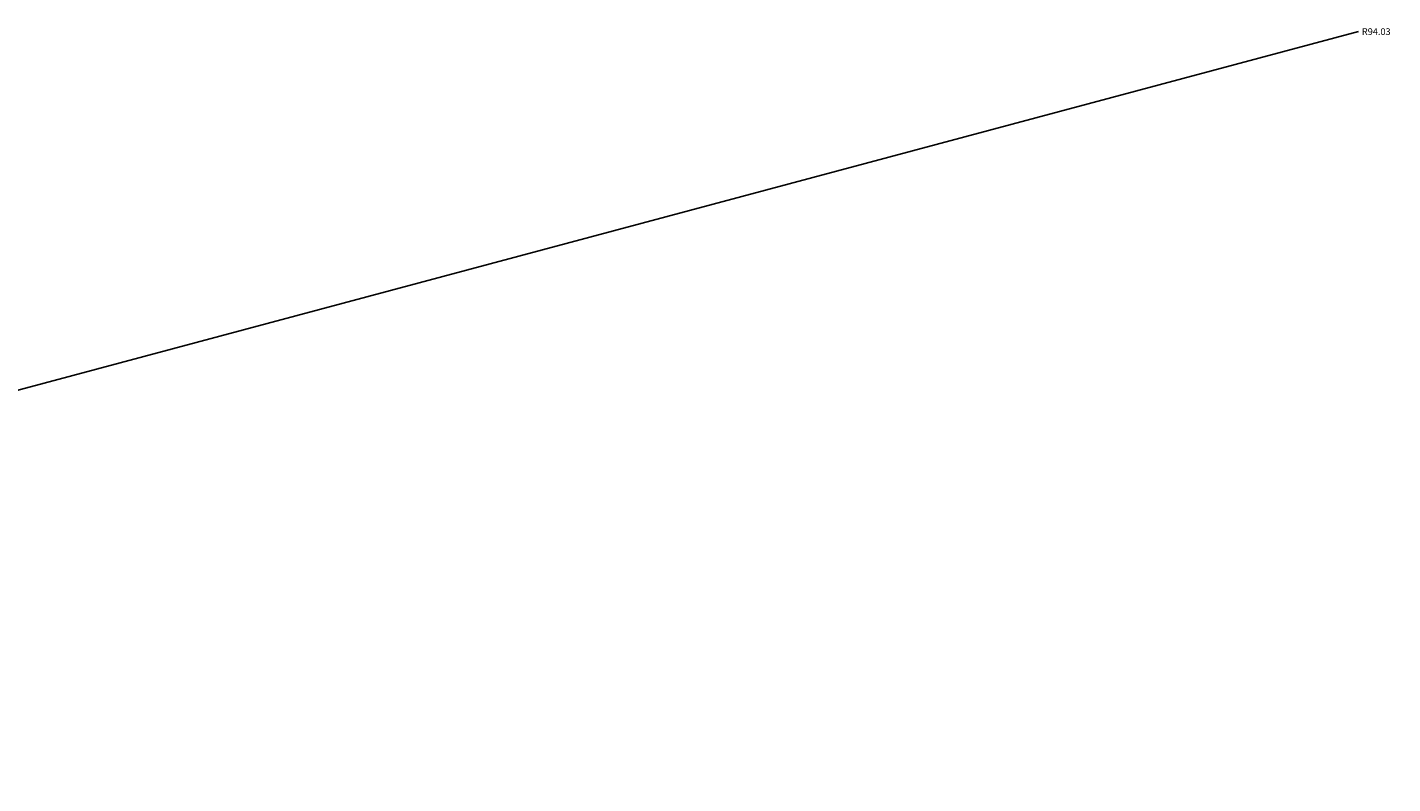
# Model space of a CAD drawing. Units: inches. Extents: x -12 to 334, y -10 to 186.
# Tile 77 of 77: x 297 to 334, y 111 to 131. Entities that reach past the tile are written whole.
import ezdxf

# ---------------------------------------------------------------- set-up
doc = ezdxf.new("R2010")
doc.units = ezdxf.units.IN
doc.header["$MEASUREMENT"] = 0
doc.layers.add('M-DIMS', color=2, linetype='Continuous', lineweight=18)
doc.styles.get("Standard").update_dxf_attribs({"font": 'arial.ttf'})
doc.dimstyles.get("Standard").update_dxf_attribs({"dimtxt": 0.18, "dimasz": 0.18, "dimexe": 0.18, "dimexo": 0.0625, "dimgap": 0.09, "dimtad": 0, "dimtih": 1, "dimtoh": 1, "dimdec": 4, "dimzin": 0, "dimdsep": 46, "dimtxsty": 'Standard', "dimcen": 0.09, "dimadec": 0, "dimazin": 0, "dimtfac": 1, "dimtdec": 4, "dimtofl": 0, "dimtmove": 0, "dimatfit": 3, "dimfxl": 1, "dimtolj": 1, "dimtzin": 0, "dimarcsym": 0})

# ---------------------------------------------------------------- blocks, each defined once
blk = doc.blocks.new('*D40')
at = {"layer": 'Defpoints', "color": 0, "transparency": 16777216}
for p in [(278.229, 116.208), (187.394, 91.899)]:
    blk.add_point(p, dxfattribs=at)
at = {"layer": 'M-DIMS', "color": 0, "lineweight": -2, "transparency": 16777216}
for p, q in [((332.73, 130.793), (278.403, 116.254)), ((187.304, 91.899), (187.484, 91.899)), ((187.394, 91.809), (187.394, 91.989))]:
    blk.add_line(p, q, dxfattribs=at)
at = {"layer": 'M-DIMS', "color": 0, "transparency": 16777216}
blk.add_solid([(278.395, 116.283), (278.411, 116.225), (278.229, 116.208)], dxfattribs=at)
at = {"layer": 'M-DIMS', "color": 0, "transparency": 16777216, "insert": (333.21, 130.793), "char_height": 0.18, "attachment_point": 5}
blk.add_mtext('\\A1;R94.03', dxfattribs=at)

msp = doc.modelspace()

# ---------------------------------------------------------------- dimensions: what is measured, and where the dimension line sits
at = {"layer": 'M-DIMS'}
dim = msp.add_radius_dim(center=(187.3936, 91.8988), mpoint=(278.2291, 116.2078), dimstyle='Standard', override={"dimdec": 2, "dimlfac": 1, "dimrnd": 0, "dimzin": 0, "dimdsep": 46, "dimlunit": 2}, dxfattribs=at)
dim.commit()
dim.dimension.update_dxf_attribs({"geometry": '*D40', "text_midpoint": (332.7304, 130.7932), "dimtype": 164})

doc.saveas('drawing.dxf')
